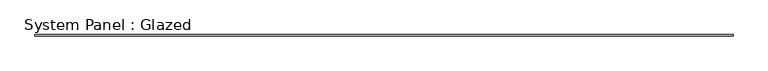
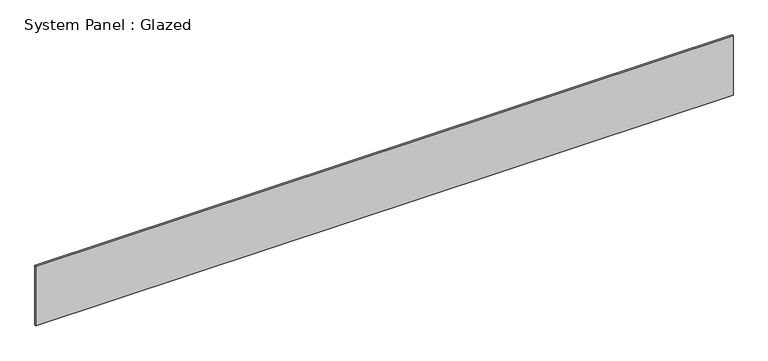
"""IFC4 building model written with IfcOpenShell, lengths in millimetres: plate geometry, System Panel : Glazed."""

from ifc_helpers import new_model, si_unit, origin, origin_with_axes, place, context, project, spatial, polyline, outline, extrude, source, transform, mapped, element, save


def system_panel_glazed_7cd9bc56(model_context):
    return source(origin(), model_context, "Body", "SweptSolid", [
        extrude(outline(polyline([(6411.1276373, 19.05), (-6411.1276373, 19.05), (-6411.1276373, 44.45), (6411.1276373, 44.45), (6411.1276373, 19.05)])), origin_with_axes(), (0.0, 0.0, 1.0), 1155.7),
    ])


if __name__ == "__main__":
    model = new_model("IFC4")
    model_context = context("Model", 3, world=origin())
    ifc_project = project(units=[si_unit("LENGTHUNIT", "METRE", prefix="MILLI")], contexts=[model_context])
    site = spatial("IfcSite", under=ifc_project)
    building = spatial("IfcBuilding", under=site)
    placement = place(None, origin())
    system_panel_glazed_shape = system_panel_glazed_7cd9bc56(model_context)
    element("IfcPlate", 1, ObjectType="System Panel : Glazed", at=placement, inside=building, context=model_context, shape_type="MappedRepresentation", body=[
        mapped(system_panel_glazed_shape, transform((0.0, 0.0, 0.0), x_axis=(1.0, 0.0, 0.0), y_axis=(0.0, 1.0, 0.0), z_axis=(0.0, 0.0, 1.0))),
    ])
    save(model, "model.ifc")

# Revit data of these elements
# Type "System Panel : Glazed"
#   Construction Type Id = "GSP4R"
#   Analytic Construction = "1/8 in Pilkington single glazing"
#   Visual Light Transmittance = 0.9
#   Solar Heat Gain Coefficient = 0.86
#   Heat Transfer Coefficient (U) = 1.18115 BTU/(h·ft²·°F)
# Element 1 (IfcPlate, "System Panel : Glazed")
#   Materials on its faces: "Glass"
# Materials
#   "Glass": class "Glass", colour RGB 0 128 192, transparency 0.75, Description = "Soda Lime Glass", Cost = 0
